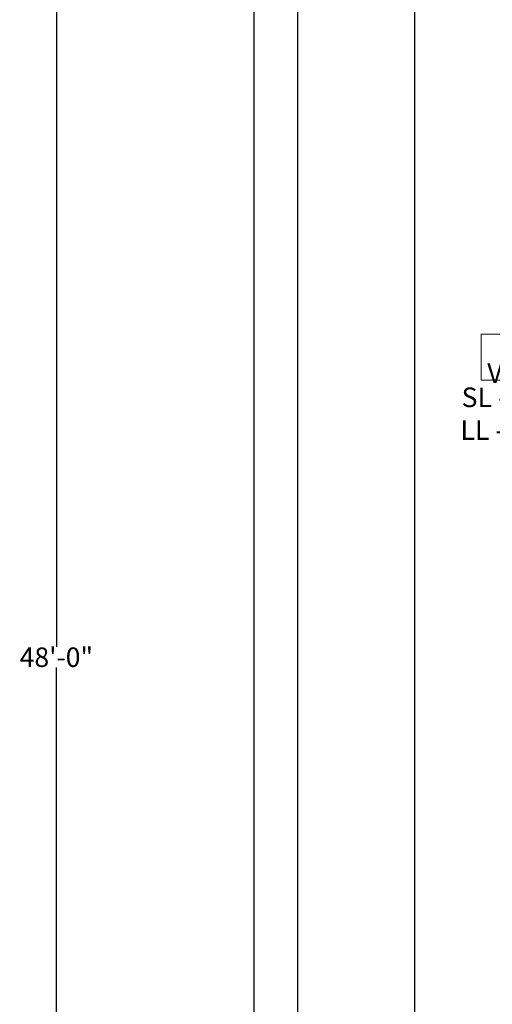
# Model space of a CAD drawing. Units: inches. Extents: x 2 to 905, y 9 to 678.
# Tile 2 of 8: x 5 to 102, y 272 to 474. Entities that reach past the tile are written whole.
import ezdxf

# ---------------------------------------------------------------- set-up
doc = ezdxf.new("R2010")
doc.units = ezdxf.units.IN
doc.layers.add('A-ANNO-DIMS', color=7, linetype='Continuous', lineweight=18)
doc.layers.add('C-PROP', color=7, linetype='Continuous', lineweight=25)
doc.layers.add('A-ANNO-IDEN', color=251, linetype='Continuous', lineweight=18, true_color=0x636466)
doc.styles.add('PDF ArialMT', font='arial.ttf')
doc.styles.get("Standard").update_dxf_attribs({"font": 'arial.ttf'})
doc.dimstyles.get("Standard").update_dxf_attribs({"dimtxt": 4, "dimasz": 4, "dimexe": 0.18, "dimexo": 0.0625, "dimgap": 0.09, "dimtad": 0, "dimtih": 1, "dimtoh": 1, "dimdec": 1, "dimzin": 0, "dimdsep": 46, "dimlunit": 3, "dimtxsty": 'Standard', "dimblk": 'ARCHTICK', "dimcen": 0, "dimse1": 1, "dimse2": 1, "dimclrt": 1, "dimadec": 0, "dimazin": 0, "dimtfac": 1, "dimtdec": 1, "dimtofl": 0, "dimtmove": 0, "dimatfit": 3, "dimfxl": 1, "dimtolj": 1, "dimtzin": 0, "dimarcsym": 0})

# ---------------------------------------------------------------- blocks, each defined once
blk = doc.blocks.new('_ArchTick')
at = {"color": 0, "linetype": 'ByBlock', "const_width": 0.15}
blk.add_lwpolyline([(-0.5, -0.5), (0.5, 0.5)], dxfattribs=at)
blk = doc.blocks.new('*D98')
at = {"layer": 'A-ANNO-DIMS', "color": 0, "lineweight": -2, "transparency": 16777216}
for p, q in [((116.91, 413.58), (116.91, 403.71)), ((116.91, 389.58), (116.91, 399.45))]:
    blk.add_line(p, q, dxfattribs=at)
at = {"layer": 'Defpoints', "color": 0, "transparency": 16777216}
for p in [(116.91, 413.58), (120.51, 413.58), (120.51, 389.58)]:
    blk.add_point(p, dxfattribs=at)
at = {"layer": 'A-ANNO-DIMS', "color": 0, "lineweight": -2, "transparency": 16777216, "xscale": 4, "yscale": 4, "zscale": 4}
for p, rotation in [((116.91, 413.58), 90), ((116.91, 389.58), 270)]:
    blk.add_blockref('_ArchTick', p, dxfattribs=dict(at, rotation=rotation))
at = {"layer": 'A-ANNO-DIMS', "color": 1, "transparency": 16777216, "insert": (116.91, 401.58), "char_height": 4, "attachment_point": 5}
blk.add_mtext('\\A1;V2 2\'-0" TYP.', dxfattribs=at)
blk = doc.blocks.new('*D103')
at = {"layer": 'A-ANNO-DIMS', "color": 0, "lineweight": -2, "transparency": 16777216}
for p, q in [((12.45, 631.22), (12.45, 345.35)), ((12.45, 55.22), (12.45, 341.09))]:
    blk.add_line(p, q, dxfattribs=at)
at = {"layer": 'Defpoints', "color": 0, "transparency": 16777216}
for p in [(12.45, 631.22), (53.05, 631.22), (53.05, 55.22)]:
    blk.add_point(p, dxfattribs=at)
at = {"layer": 'A-ANNO-DIMS', "color": 0, "lineweight": -2, "transparency": 16777216, "xscale": 4, "yscale": 4, "zscale": 4}
for p, rotation in [((12.45, 631.22), 90), ((12.45, 55.22), 270)]:
    blk.add_blockref('_ArchTick', p, dxfattribs=dict(at, rotation=rotation))
at = {"layer": 'A-ANNO-DIMS', "color": 1, "transparency": 16777216, "insert": (12.45, 343.22), "char_height": 4, "attachment_point": 5}
blk.add_mtext('\\A1;48\'-0"', dxfattribs=at)
blk = doc.blocks.new('*D107')
at = {"layer": 'A-ANNO-DIMS', "color": 0, "lineweight": -2, "transparency": 16777216}
for p, q in [((62.05, 14.62), (68.61, 14.62)), ((86.05, 14.62), (79.49, 14.62))]:
    blk.add_line(p, q, dxfattribs=at)
at = {"layer": 'Defpoints', "color": 0, "transparency": 16777216}
for p in [(62.05, 622.22), (86.05, 598.22), (86.05, 14.62)]:
    blk.add_point(p, dxfattribs=at)
at = {"layer": 'A-ANNO-DIMS', "color": 0, "lineweight": -2, "transparency": 16777216, "xscale": 4, "yscale": 4, "zscale": 4, "rotation": 180}
blk.add_blockref('_ArchTick', (62.05, 14.62), dxfattribs=at)
at = {"layer": 'A-ANNO-DIMS', "color": 0, "lineweight": -2, "transparency": 16777216, "xscale": 4, "yscale": 4, "zscale": 4}
blk.add_blockref('_ArchTick', (86.05, 14.62), dxfattribs=at)
at = {"layer": 'A-ANNO-DIMS', "color": 1, "transparency": 16777216, "insert": (74.05, 14.62), "char_height": 4, "attachment_point": 5}
blk.add_mtext('\\A1;2\'-0"', dxfattribs=at)

msp = doc.modelspace()

# ---------------------------------------------------------------- linework, layer by layer
at = {"layer": 'A-ANNO-IDEN'}
msp.add_lwpolyline([(99.78, 409.64), (112.68, 409.64), (112.68, 400.16), (99.78, 400.16)], close=True, dxfattribs=at)
at = {"layer": 'C-PROP'}
msp.add_lwpolyline([(857.05, 535.22), (857.05, 631.22), (53.05, 631.22), (53.05, 55.22), (857.05, 55.22), (857.05, 355.22), (848.05, 355.22), (848.05, 64.22), (62.05, 64.22), (62.05, 622.22), (848.05, 622.22), (848.05, 535.22)], close=True, dxfattribs=at)
msp.add_lwpolyline([(848.05, 598.22), (86.05, 598.22), (86.05, 88.22), (824.05, 88.22), (824.05, 355.22), (836.05, 355.22), (848.05, 355.22)], dxfattribs=at)

# ---------------------------------------------------------------- texts
at = {"layer": 'A-ANNO-IDEN', "char_height": 4.023, "attachment_point": 4, "style": 'PDF ArialMT'}
for s, insert in [('SL - 7\'0"', (95.72, 396.11)), ('LL - 9\'0"', (95.49, 389.38))]:
    msp.add_mtext(s, dxfattribs=dict(at, insert=insert))

# ---------------------------------------------------------------- dimensions: what is measured, and where the dimension line sits
at = {"layer": 'A-ANNO-DIMS'}
dim = msp.add_linear_dim(base=(12.45, 631.22), p1=(53.05, 55.22), p2=(53.05, 631.22), angle=90, dimstyle='Standard', override={"dimdec": 1, "dimlfac": 1, "dimrnd": 0, "dimzin": 1, "dimdsep": 46, "dimlunit": 4, "dimfrac": 2}, dxfattribs=at)
dim.commit()
dim.dimension.update_dxf_attribs({"geometry": '*D103', "text_midpoint": (12.45, 343.22)})
dim = msp.add_linear_dim(base=(86.05, 14.62), p1=(62.05, 622.22), p2=(86.05, 598.22), dimstyle='Standard', override={"dimdec": 1, "dimlfac": 1, "dimrnd": 0, "dimzin": 1, "dimdsep": 46, "dimlunit": 4, "dimfrac": 2}, dxfattribs=at)
dim.commit()
dim.dimension.update_dxf_attribs({"geometry": '*D107', "text_midpoint": (74.05, 14.62)})
dim = msp.add_linear_dim(base=(116.91, 413.58), p1=(120.51, 389.58), p2=(120.51, 413.58), angle=90, text='V2 <> TYP.', dimstyle='Standard', override={"dimdec": 1, "dimlfac": 1, "dimrnd": 0, "dimzin": 1, "dimdsep": 46, "dimlunit": 4, "dimfrac": 2}, dxfattribs=at)
dim.commit()
dim.dimension.update_dxf_attribs({"geometry": '*D98', "text_midpoint": (116.91, 401.58)})

doc.saveas('drawing.dxf')
